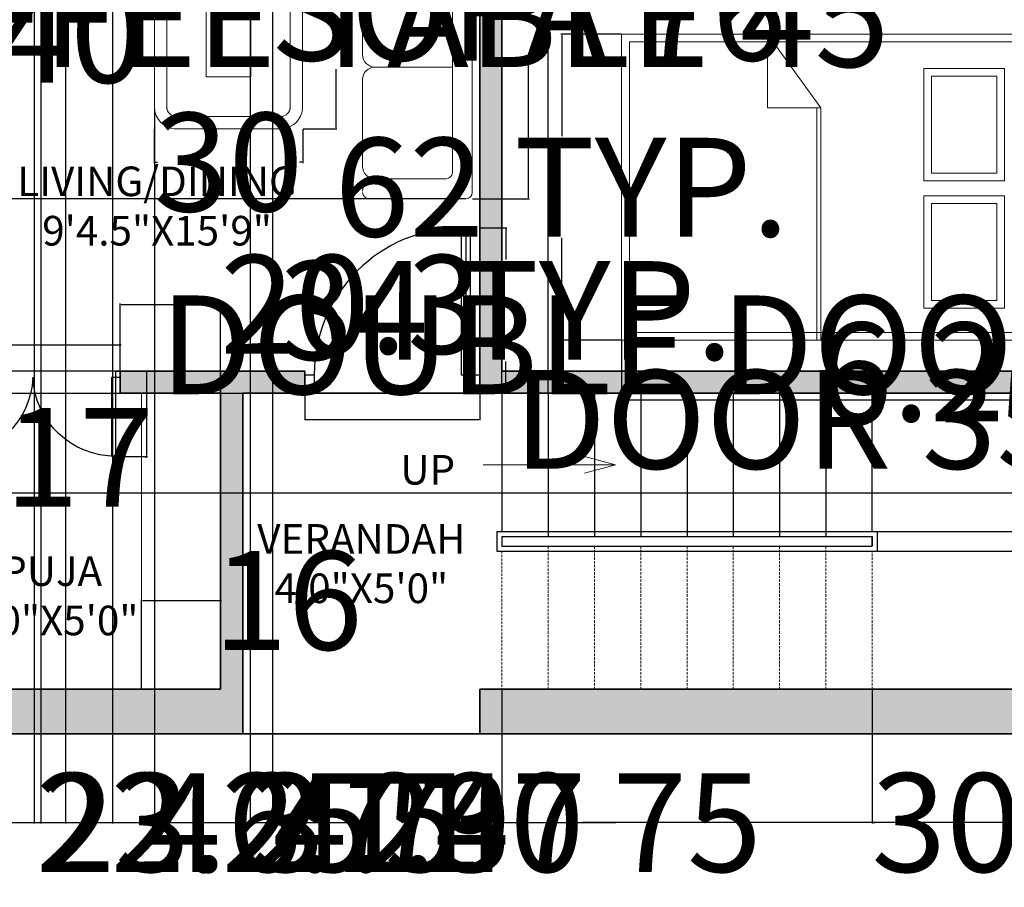
# Model space of a CAD drawing. Units: inches. Extents: x 305 to 776, y 38 to 479.
# Tile 8 of 14: x 419 to 618, y 38 to 214. Entities that reach past the tile are written whole.
import ezdxf

# ---------------------------------------------------------------- set-up
doc = ezdxf.new("R2010")
doc.units = ezdxf.units.IN
doc.header["$MEASUREMENT"] = 0
doc.linetypes.add('DASHED', pattern=[0.75, 0.5, -0.25])
for name, color, linetype, lineweight in [('A-ANNO-DIMS', 2, 'Continuous', 18), ('A-ANNO-SYMB', 3, 'Continuous', 18), ('A-AREA-IDEN', 7, 'Continuous', 18), ('A-DOOR', 4, 'Continuous', 25), ('A-FLOR-CASE', 8, 'Continuous', 20), ('A-FLOR-STRS', 7, 'Continuous', 25), ('A-FLOR-STRS-OVHD', 7, 'DASHED', 18), ('A-FURN', 8, 'Continuous', 18), ('A-WALL', 7, 'Continuous', 35), ('A-WALL-PATT', 252, 'Continuous', 13)]:
    doc.layers.add(name, color=color, linetype=linetype, lineweight=lineweight)
doc.styles.get("Standard").update_dxf_attribs({"font": 'arial.ttf'})
doc.dimstyles.get("Standard").update_dxf_attribs({"dimtxt": 20, "dimasz": 0.18, "dimexe": 0.18, "dimexo": 0.0625, "dimgap": 0.09, "dimtad": 0, "dimtih": 1, "dimtoh": 1, "dimdec": 4, "dimzin": 0, "dimdsep": 46, "dimtxsty": 'Standard', "dimcen": 0.09, "dimadec": 0, "dimazin": 0, "dimtfac": 1, "dimtdec": 4, "dimtofl": 0, "dimtmove": 0, "dimatfit": 3, "dimfxl": 1, "dimtolj": 1, "dimtzin": 0, "dimarcsym": 0})

# ---------------------------------------------------------------- blocks, each defined once
blk = doc.blocks.new('A$C296830DC')
blk.add_line((828.9, 852.6), (828.9, 94.7))
for points in [[(852.6, 94.7), (852.6, 852.6), (805.3, 852.6), (805.3, 94.7)], [(47.4, 94.7), (47.4, 0), (0, 0), (0, 94.7)], [(900, 94.7), (900, 0), (852.6, 0), (852.6, 94.7)]]:
    blk.add_lwpolyline(points, close=True)
blk.add_arc((805.3, 94.7), 757.9, 90, 180)
blk = doc.blocks.new('BED')
for p, q in [((1579.44, 254.58), (1564.49, 243.77)), ((1564.49, 243.77), (1579.44, 254.58)), ((1626.49, 254.58), (1579.44, 254.58)), ((1579.44, 254.58), (1579.44, 243.77)), ((1626.49, 253.76), (1579.44, 253.76)), ((1579.44, 243.77), (1564.49, 243.77))]:
    blk.add_line(p, q)
for points in [[(1626.49, 214.2), (1564.49, 214.2), (1564.49, 294.96), (1626.49, 294.96)], [(1624.92, 215.77), (1566.06, 215.77), (1566.06, 293.39), (1624.92, 293.39)], [(1594.24, 275.39), (1571.42, 275.39), (1571.42, 291.78), (1594.24, 291.78)], [(1620.04, 275.39), (1597.22, 275.39), (1597.22, 291.78), (1620.04, 291.78)], [(1592.67, 276.96), (1572.99, 276.96), (1572.99, 290.21), (1592.67, 290.21)], [(1618.47, 276.96), (1598.79, 276.96), (1598.79, 290.21), (1618.47, 290.21)]]:
    blk.add_lwpolyline(points, close=True)
blk = doc.blocks.new('sofa-25')
at = {"color": 0, "linetype": 'ByBlock'}
for p, q in [((0.5351, 0.5197), (0.124, 0.5197)), ((1.0702, 0.5197), (0.6532, 0.5197)), ((1.5935, 0.5197), (1.1883, 0.5197)), ((-0.0295, 0.0295), (-0.0295, 0.4902)), ((1.7471, 0.0591), (1.7471, 0.4902)), ((0.065, 0.124), (0.065, 0.4607)), ((0.5942, 0.0945), (0.5942, 0.4607)), ((1.1293, 0.0945), (1.1293, 0.4607)), ((1.6526, 0.1181), (1.6526, 0.4607)), ((0.0945, 0.0945), (1.6289, 0.0945)), ((0, 0), (1.688, 0))]:
    blk.add_line(p, q, dxfattribs=at)
for centre, radius, start, end in [((0, 0.4902), 0.0295, 90, 180), ((0.0059, 0.4607), 0.0591, 0, 90), ((0.124, 0.4607), 0.0591, 90, 180), ((0.5351, 0.4607), 0.0591, 0, 90), ((0.6532, 0.4607), 0.0591, 90, 180), ((1.0702, 0.4607), 0.0591, 0, 90), ((1.1883, 0.4607), 0.0591, 90, 180), ((1.5935, 0.4607), 0.0591, 0, 90), ((1.7116, 0.4607), 0.0591, 90, 180), ((1.7175, 0.4902), 0.0295, 0, 90), ((0.0945, 0.124), 0.0295, 180, 270), ((1.6289, 0.1181), 0.0236, 270, 0), ((1.688, 0.0591), 0.0591, 270, 0), ((0, 0.0295), 0.0295, 180, 270)]:
    blk.add_arc(centre, radius, start, end, dxfattribs=at)
blk = doc.blocks.new('carp')
for p, q in [((853.97, 318.32), (853.97, 318.33)), ((857.97, 314.33), (857.96, 314.33))]:
    blk.add_line(p, q)
for points in [[(853.97, 318.33), (831.57, 318.33)], [(853.97, 315.83), (831.57, 315.83)], [(827.97, 314.73), (827.97, 277.33)], [(830.47, 314.73), (830.47, 277.33)], [(855.47, 277.33), (855.47, 314.33)], [(857.97, 277.33), (857.97, 314.33)], [(831.97, 275.83), (853.97, 275.83)], [(831.97, 273.33), (853.97, 273.33)]]:
    blk.add_lwpolyline(points)
blk.add_lwpolyline([(838.47, 307.83), (838.47, 283.83), (847.47, 283.83), (847.47, 307.83)], close=True)
for centre, radius, start, end in [((831.77, 314.53), 3.81, 87.0112, 182.9888), ((853.86, 314.21), 4.11, 358.8861, 88.4626), ((831.77, 314.53), 1.31, 87.0112, 182.9888), ((853.86, 314.21), 1.61, 358.8861, 88.4626), ((832.52, 277.88), 4.59, 186.916, 263.084), ((832.52, 277.88), 2.09, 186.916, 263.084), ((853.42, 277.88), 2.09, 276.916, 353.084), ((853.42, 277.88), 4.59, 276.916, 353.084)]:
    blk.add_arc(centre, radius, start, end)
blk = doc.blocks.new('A$C16FA5A5B')
for p, q in [((50, 487.5), (25, 487.5)), ((25, 487.5), (25, 37.5)), ((50, 37.5), (50, 487.5)), ((950, 37.5), (950, 487.5)), ((950, 487.5), (975, 487.5)), ((975, 487.5), (975, 37.5)), ((0, 0), (0, 37.5)), ((0, 37.5), (25, 37.5)), ((25, 0), (0, 0)), ((25, 37.5), (25, 0)), ((25, 37.5), (50, 37.5)), ((975, 37.5), (950, 37.5)), ((975, 37.5), (975, 0)), ((1000, 37.5), (975, 37.5)), ((975, 0), (1000, 0)), ((1000, 0), (1000, 37.5))]:
    blk.add_line(p, q)
for centre, start, end in [((28.6, 15.6), 2.662, 90.4344), ((971.4, 15.6), 89.5656, 177.338)]:
    blk.add_arc(centre, 471.9, start, end)
blk = doc.blocks.new('*D17')
at = {"layer": 'A-ANNO-DIMS', "color": 0, "lineweight": -2, "transparency": 16777216}
for p, q in [((476.73, 138.32), (476.73, 132.89)), ((512.13, 138.32), (512.13, 132.89)), ((476.91, 133.07), (511.95, 133.07)), ((512.13, 133.07), (512.31, 133.07))]:
    blk.add_line(p, q, dxfattribs=at)
at = {"layer": 'A-ANNO-DIMS', "color": 0, "transparency": 16777216}
for points in [[(476.91, 133.1), (476.91, 133.04), (476.73, 133.07)], [(511.95, 133.1), (511.95, 133.04), (512.13, 133.07)]]:
    blk.add_solid(points, dxfattribs=at)
at = {"layer": 'Defpoints', "color": 0, "transparency": 16777216}
for p in [(476.73, 138.38), (512.13, 138.38), (512.13, 133.07)]:
    blk.add_point(p, dxfattribs=at)
at = {"layer": 'A-ANNO-DIMS', "color": 0, "transparency": 16777216, "insert": (606.37, 133.07), "char_height": 20, "attachment_point": 5}
blk.add_mtext('\\A1;DOOR 35 TYP.', dxfattribs=at)
blk = doc.blocks.new('*D18')
at = {"layer": 'A-ANNO-DIMS', "color": 0, "lineweight": -2, "transparency": 16777216}
for p, q in [((512.2, 171.92), (517.62, 171.92)), ((517.44, 171.74), (517.44, 165.46)), ((517.44, 138.56), (517.44, 144.84)), ((512.2, 138.38), (517.62, 138.38))]:
    blk.add_line(p, q, dxfattribs=at)
at = {"layer": 'A-ANNO-DIMS', "color": 0, "transparency": 16777216}
for points in [[(517.41, 171.74), (517.47, 171.74), (517.44, 171.92)], [(517.41, 138.56), (517.47, 138.56), (517.44, 138.38)]]:
    blk.add_solid(points, dxfattribs=at)
at = {"layer": 'Defpoints', "color": 0, "transparency": 16777216}
for p in [(512.13, 171.92), (517.44, 171.92), (512.13, 138.38)]:
    blk.add_point(p, dxfattribs=at)
at = {"layer": 'A-ANNO-DIMS', "color": 0, "transparency": 16777216, "insert": (517.44, 155.15), "char_height": 20, "attachment_point": 5}
blk.add_mtext('\\A1;34 TYP.', dxfattribs=at)
blk = doc.blocks.new('*D19')
at = {"layer": 'A-ANNO-DIMS', "color": 0, "lineweight": -2, "transparency": 16777216}
for p, q in [((557.63, 250.82), (557.63, 245.98)), ((589.13, 250.82), (589.13, 245.98)), ((557.63, 246.16), (557.45, 246.16)), ((588.95, 246.16), (557.81, 246.16))]:
    blk.add_line(p, q, dxfattribs=at)
at = {"layer": 'A-ANNO-DIMS', "color": 0, "transparency": 16777216}
for points in [[(557.81, 246.19), (557.81, 246.13), (557.63, 246.16)], [(588.95, 246.19), (588.95, 246.13), (589.13, 246.16)]]:
    blk.add_solid(points, dxfattribs=at)
at = {"layer": 'Defpoints', "color": 0, "transparency": 16777216}
for p in [(557.63, 250.88), (589.13, 250.88), (557.63, 246.16)]:
    blk.add_point(p, dxfattribs=at)
at = {"layer": 'A-ANNO-DIMS', "color": 0, "transparency": 16777216, "insert": (463.39, 246.16), "char_height": 20, "attachment_point": 5}
blk.add_mtext('\\A1;DOOR 32 TYP.', dxfattribs=at)
blk = doc.blocks.new('*D21')
at = {"layer": 'A-ANNO-DIMS', "color": 0, "lineweight": -2, "transparency": 16777216}
for p, q in [((403.93, 142.94), (403.93, 148.37)), ((404.11, 148.19), (439.15, 148.19)), ((439.33, 142.94), (439.33, 148.37)), ((439.33, 148.19), (439.51, 148.19))]:
    blk.add_line(p, q, dxfattribs=at)
at = {"layer": 'A-ANNO-DIMS', "color": 0, "transparency": 16777216}
for points in [[(404.11, 148.22), (404.11, 148.16), (403.93, 148.19)], [(439.15, 148.22), (439.15, 148.16), (439.33, 148.19)]]:
    blk.add_solid(points, dxfattribs=at)
at = {"layer": 'Defpoints', "color": 0, "transparency": 16777216}
for p in [(439.33, 148.19), (403.93, 142.88), (439.33, 142.88)]:
    blk.add_point(p, dxfattribs=at)
at = {"layer": 'A-ANNO-DIMS', "color": 0, "transparency": 16777216, "insert": (560.63, 148.19), "char_height": 20, "attachment_point": 5}
blk.add_mtext('\\A1;DOUBLE DOOR 35', dxfattribs=at)
blk = doc.blocks.new('*D22')
at = {"layer": 'A-ANNO-DIMS', "color": 0, "lineweight": -2, "transparency": 16777216}
for p, q in [((439.4, 142.88), (444.82, 142.88)), ((444.64, 142.7), (444.64, 125.74)), ((439.4, 125.56), (444.82, 125.56)), ((444.64, 125.38), (444.46, 125.38)), ((444.64, 125.56), (444.64, 125.38))]:
    blk.add_line(p, q, dxfattribs=at)
at = {"layer": 'A-ANNO-DIMS', "color": 0, "transparency": 16777216}
for points in [[(444.61, 142.7), (444.67, 142.7), (444.64, 142.88)], [(444.61, 125.74), (444.67, 125.74), (444.64, 125.56)]]:
    blk.add_solid(points, dxfattribs=at)
at = {"layer": 'Defpoints', "color": 0, "transparency": 16777216}
for p in [(439.33, 142.88), (439.33, 125.56), (444.64, 125.56)]:
    blk.add_point(p, dxfattribs=at)
at = {"layer": 'A-ANNO-DIMS', "color": 0, "transparency": 16777216, "insert": (430.99, 125.38), "char_height": 20, "attachment_point": 5}
blk.add_mtext('\\A1;17', dxfattribs=at)
blk = doc.blocks.new('*D29')
at = {"layer": 'A-ANNO-DIMS', "color": 0, "lineweight": -2, "transparency": 16777216}
for p, q in [((540.87, 149.08), (540.87, 136.85)), ((621.63, 149.08), (621.63, 136.85)), ((541.05, 137.03), (621.45, 137.03)), ((621.63, 137.03), (621.81, 137.03))]:
    blk.add_line(p, q, dxfattribs=at)
at = {"layer": 'A-ANNO-DIMS', "color": 0, "transparency": 16777216}
for points in [[(541.05, 137.06), (541.05, 137), (540.87, 137.03)], [(621.45, 137.06), (621.45, 137), (621.63, 137.03)]]:
    blk.add_solid(points, dxfattribs=at)
at = {"layer": 'Defpoints', "color": 0, "transparency": 16777216}
for p in [(540.87, 149.14), (621.63, 149.14), (621.63, 137.03)]:
    blk.add_point(p, dxfattribs=at)
at = {"layer": 'A-ANNO-DIMS', "color": 0, "transparency": 16777216, "insert": (702.74, 137.03), "char_height": 20, "attachment_point": 5}
blk.add_mtext('\\A1;BED 81 TYP.', dxfattribs=at)
blk = doc.blocks.new('*D30')
at = {"layer": 'A-ANNO-DIMS', "color": 0, "lineweight": -2, "transparency": 16777216}
for p, q in [((540.81, 211.14), (528.58, 211.14)), ((528.76, 210.96), (528.76, 190.45)), ((528.76, 149.32), (528.76, 169.84)), ((540.81, 149.14), (528.58, 149.14))]:
    blk.add_line(p, q, dxfattribs=at)
at = {"layer": 'A-ANNO-DIMS', "color": 0, "transparency": 16777216}
for points in [[(528.73, 210.96), (528.79, 210.96), (528.76, 211.14)], [(528.73, 149.32), (528.79, 149.32), (528.76, 149.14)]]:
    blk.add_solid(points, dxfattribs=at)
at = {"layer": 'Defpoints', "color": 0, "transparency": 16777216}
for p in [(540.87, 211.14), (528.76, 149.14), (540.87, 149.14)]:
    blk.add_point(p, dxfattribs=at)
at = {"layer": 'A-ANNO-DIMS', "color": 0, "transparency": 16777216, "insert": (528.76, 180.14), "char_height": 20, "attachment_point": 5}
blk.add_mtext('\\A1;62 TYP.', dxfattribs=at)
blk = doc.blocks.new('*D35')
at = {"layer": 'A-ANNO-DIMS', "color": 0, "lineweight": -2, "transparency": 16777216}
for p, q in [((510.7, 253.8), (522.21, 253.8)), ((522.03, 253.62), (522.03, 226.23)), ((522.03, 177.97), (522.03, 205.36)), ((510.7, 177.79), (522.21, 177.79))]:
    blk.add_line(p, q, dxfattribs=at)
at = {"layer": 'A-ANNO-DIMS', "color": 0, "transparency": 16777216}
for points in [[(522, 253.62), (522.06, 253.62), (522.03, 253.8)], [(522, 177.97), (522.06, 177.97), (522.03, 177.79)]]:
    blk.add_solid(points, dxfattribs=at)
at = {"layer": 'Defpoints', "color": 0, "transparency": 16777216}
for p in [(510.63, 253.8), (522.03, 253.8), (510.63, 177.79)]:
    blk.add_point(p, dxfattribs=at)
at = {"layer": 'A-ANNO-DIMS', "color": 0, "transparency": 16777216, "insert": (522.03, 215.8), "char_height": 20, "attachment_point": 5}
blk.add_mtext('\\A1;SOFA 76', dxfattribs=at)
blk = doc.blocks.new('*D37')
at = {"layer": 'A-ANNO-DIMS', "color": 0, "lineweight": -2, "transparency": 16777216}
for p, q in [((476.35, 237.03), (483.22, 237.03)), ((483.04, 236.85), (483.04, 224.94)), ((483.04, 192.15), (483.04, 204.06)), ((476.35, 191.97), (483.22, 191.97))]:
    blk.add_line(p, q, dxfattribs=at)
at = {"layer": 'A-ANNO-DIMS', "color": 0, "transparency": 16777216}
for points in [[(483.01, 236.85), (483.07, 236.85), (483.04, 237.03)], [(483.01, 192.15), (483.07, 192.15), (483.04, 191.97)]]:
    blk.add_solid(points, dxfattribs=at)
at = {"layer": 'Defpoints', "color": 0, "transparency": 16777216}
for p in [(476.28, 237.03), (483.04, 237.03), (476.28, 191.97)]:
    blk.add_point(p, dxfattribs=at)
at = {"layer": 'A-ANNO-DIMS', "color": 0, "transparency": 16777216, "insert": (483.04, 214.5), "char_height": 20, "attachment_point": 5}
blk.add_mtext('\\A1;COFFEE TABLE 45', dxfattribs=at)
blk = doc.blocks.new('*D38')
at = {"layer": 'A-ANNO-DIMS', "color": 0, "lineweight": -2, "transparency": 16777216}
for p, q in [((446.19, 191.91), (446.19, 185.03)), ((476.28, 191.91), (476.28, 185.03)), ((446.37, 185.21), (446.86, 185.21)), ((476.1, 185.21), (475.61, 185.21))]:
    blk.add_line(p, q, dxfattribs=at)
at = {"layer": 'A-ANNO-DIMS', "color": 0, "transparency": 16777216}
for points in [[(446.37, 185.24), (446.37, 185.18), (446.19, 185.21)], [(476.1, 185.24), (476.1, 185.18), (476.28, 185.21)]]:
    blk.add_solid(points, dxfattribs=at)
at = {"layer": 'Defpoints', "color": 0, "transparency": 16777216}
for p in [(446.19, 191.97), (476.28, 191.97), (476.28, 185.21)]:
    blk.add_point(p, dxfattribs=at)
at = {"layer": 'A-ANNO-DIMS', "color": 0, "transparency": 16777216, "insert": (461.24, 185.21), "char_height": 20, "attachment_point": 5}
blk.add_mtext('\\A1;30', dxfattribs=at)
blk = doc.blocks.new('*D39')
at = {"layer": 'A-ANNO-DIMS', "color": 0, "lineweight": -2, "transparency": 16777216}
for p, q in [((404.2, 231.29), (410.31, 231.29)), ((410.13, 231.11), (410.13, 221.59)), ((410.13, 191.47), (410.13, 200.99)), ((404.2, 191.29), (410.31, 191.29))]:
    blk.add_line(p, q, dxfattribs=at)
at = {"layer": 'A-ANNO-DIMS', "color": 0, "transparency": 16777216}
for points in [[(410.1, 231.11), (410.16, 231.11), (410.13, 231.29)], [(410.1, 191.47), (410.16, 191.47), (410.13, 191.29)]]:
    blk.add_solid(points, dxfattribs=at)
at = {"layer": 'Defpoints', "color": 0, "transparency": 16777216}
for p in [(404.13, 231.29), (410.13, 231.29), (404.13, 191.29)]:
    blk.add_point(p, dxfattribs=at)
at = {"layer": 'A-ANNO-DIMS', "color": 0, "transparency": 16777216, "insert": (410.13, 211.29), "char_height": 20, "attachment_point": 5}
blk.add_mtext('\\A1;TV 40', dxfattribs=at)
blk = doc.blocks.new('*D45')
at = {"layer": 'A-ANNO-DIMS', "color": 0, "lineweight": -2, "transparency": 16777216}
for p, q in [((390.63, 69.32), (390.63, 51.2)), ((630.63, 69.32), (630.63, 51.2)), ((390.81, 51.38), (488.31, 51.38)), ((630.45, 51.38), (532.95, 51.38))]:
    blk.add_line(p, q, dxfattribs=at)
at = {"layer": 'A-ANNO-DIMS', "color": 0, "transparency": 16777216}
for points in [[(390.81, 51.41), (390.81, 51.35), (390.63, 51.38)], [(630.45, 51.41), (630.45, 51.35), (630.63, 51.38)]]:
    blk.add_solid(points, dxfattribs=at)
at = {"layer": 'Defpoints', "color": 0, "transparency": 16777216}
for p in [(390.63, 69.38), (630.63, 69.38), (630.63, 51.38)]:
    blk.add_point(p, dxfattribs=at)
at = {"layer": 'A-ANNO-DIMS', "color": 0, "transparency": 16777216, "insert": (510.63, 51.38), "char_height": 20, "attachment_point": 5}
blk.add_mtext('\\A1;240', dxfattribs=at)
blk = doc.blocks.new('*D47')
at = {"layer": 'A-ANNO-DIMS', "color": 0, "lineweight": -2, "transparency": 16777216}
for p, q in [((465.63, 331.82), (465.63, 51.2)), ((470.13, 331.82), (470.13, 51.2)), ((465.81, 51.38), (469.95, 51.38)), ((470.13, 51.38), (470.31, 51.38))]:
    blk.add_line(p, q, dxfattribs=at)
at = {"layer": 'A-ANNO-DIMS', "color": 0, "transparency": 16777216}
for points in [[(465.81, 51.41), (465.81, 51.35), (465.63, 51.38)], [(469.95, 51.41), (469.95, 51.35), (470.13, 51.38)]]:
    blk.add_solid(points, dxfattribs=at)
at = {"layer": 'Defpoints', "color": 0, "transparency": 16777216}
for p in [(465.63, 331.88), (470.13, 331.88), (470.13, 51.38)]:
    blk.add_point(p, dxfattribs=at)
at = {"layer": 'A-ANNO-DIMS', "color": 0, "transparency": 16777216, "insert": (489.09, 51.38), "char_height": 20, "attachment_point": 5}
blk.add_mtext('\\A1;4.5', dxfattribs=at)
blk = doc.blocks.new('*D48')
at = {"layer": 'A-ANNO-DIMS', "color": 0, "lineweight": -2, "transparency": 16777216}
for p, q in [((404, 138.38), (648.81, 138.38)), ((648.63, 138.38), (648.63, 138.56)), ((648.63, 138.56), (648.81, 138.56)), ((648.63, 118.36), (648.63, 138.2)), ((399.7, 118.18), (648.81, 118.18))]:
    blk.add_line(p, q, dxfattribs=at)
at = {"layer": 'A-ANNO-DIMS', "color": 0, "transparency": 16777216}
for points in [[(648.6, 138.2), (648.66, 138.2), (648.63, 138.38)], [(648.6, 118.36), (648.66, 118.36), (648.63, 118.18)]]:
    blk.add_solid(points, dxfattribs=at)
at = {"layer": 'Defpoints', "color": 0, "transparency": 16777216}
for p in [(403.93, 138.38), (648.63, 138.38), (399.63, 118.18)]:
    blk.add_point(p, dxfattribs=at)
at = {"layer": 'A-ANNO-DIMS', "color": 0, "transparency": 16777216, "insert": (674.95, 138.56), "char_height": 20, "attachment_point": 5}
blk.add_mtext('\\A1;20.2', dxfattribs=at)
blk = doc.blocks.new('*D55')
at = {"layer": 'A-ANNO-DIMS', "color": 0, "lineweight": -2, "transparency": 16777216}
for p, q in [((516.63, 78.32), (516.63, 51.2)), ((591.63, 78.32), (591.63, 51.2)), ((516.81, 51.38), (539.73, 51.38)), ((591.45, 51.38), (568.54, 51.38))]:
    blk.add_line(p, q, dxfattribs=at)
at = {"layer": 'A-ANNO-DIMS', "color": 0, "transparency": 16777216}
for points in [[(516.81, 51.41), (516.81, 51.35), (516.63, 51.38)], [(591.45, 51.41), (591.45, 51.35), (591.63, 51.38)]]:
    blk.add_solid(points, dxfattribs=at)
at = {"layer": 'Defpoints', "color": 0, "transparency": 16777216}
for p in [(516.63, 78.38), (591.63, 78.38), (591.63, 51.38)]:
    blk.add_point(p, dxfattribs=at)
at = {"layer": 'A-ANNO-DIMS', "color": 0, "transparency": 16777216, "insert": (554.13, 51.38), "char_height": 20, "attachment_point": 5}
blk.add_mtext('\\A1;75', dxfattribs=at)
blk = doc.blocks.new('*D56')
at = {"layer": 'A-ANNO-DIMS', "color": 0, "lineweight": -2, "transparency": 16777216}
for p, q in [((591.63, 78.32), (591.63, 51.2)), ((621.63, 78.32), (621.63, 51.2)), ((591.81, 51.38), (592.26, 51.38)), ((621.45, 51.38), (621.01, 51.38))]:
    blk.add_line(p, q, dxfattribs=at)
at = {"layer": 'A-ANNO-DIMS', "color": 0, "transparency": 16777216}
for points in [[(591.81, 51.41), (591.81, 51.35), (591.63, 51.38)], [(621.45, 51.41), (621.45, 51.35), (621.63, 51.38)]]:
    blk.add_solid(points, dxfattribs=at)
at = {"layer": 'Defpoints', "color": 0, "transparency": 16777216}
for p in [(591.63, 78.38), (621.63, 78.38), (621.63, 51.38)]:
    blk.add_point(p, dxfattribs=at)
at = {"layer": 'A-ANNO-DIMS', "color": 0, "transparency": 16777216, "insert": (606.63, 51.38), "char_height": 20, "attachment_point": 5}
blk.add_mtext('\\A1;30', dxfattribs=at)
blk = doc.blocks.new('*D57')
at = {"layer": 'A-ANNO-DIMS', "color": 0, "lineweight": -2, "transparency": 16777216}
for p, q in [((591.7, 138.38), (648.81, 138.38)), ((648.63, 138.2), (648.63, 134.68)), ((648.63, 110.56), (648.63, 114.08)), ((591.7, 110.38), (648.81, 110.38))]:
    blk.add_line(p, q, dxfattribs=at)
at = {"layer": 'A-ANNO-DIMS', "color": 0, "transparency": 16777216}
for points in [[(648.6, 138.2), (648.66, 138.2), (648.63, 138.38)], [(648.6, 110.56), (648.66, 110.56), (648.63, 110.38)]]:
    blk.add_solid(points, dxfattribs=at)
at = {"layer": 'Defpoints', "color": 0, "transparency": 16777216}
for p in [(591.63, 138.38), (591.63, 110.38), (648.63, 110.38)]:
    blk.add_point(p, dxfattribs=at)
at = {"layer": 'A-ANNO-DIMS', "color": 0, "transparency": 16777216, "insert": (648.63, 124.38), "char_height": 20, "attachment_point": 5}
blk.add_mtext('\\A1;28', dxfattribs=at)
blk = doc.blocks.new('*D58')
at = {"layer": 'A-ANNO-DIMS', "color": 0, "lineweight": -2, "transparency": 16777216}
for p, q in [((516.63, 138.44), (516.63, 447.56)), ((516.81, 447.38), (525.83, 447.38)), ((526.01, 138.44), (526.01, 447.56)), ((526.01, 447.38), (526.19, 447.38))]:
    blk.add_line(p, q, dxfattribs=at)
at = {"layer": 'A-ANNO-DIMS', "color": 0, "transparency": 16777216}
for points in [[(516.81, 447.41), (516.81, 447.35), (516.63, 447.38)], [(525.83, 447.41), (525.83, 447.35), (526.01, 447.38)]]:
    blk.add_solid(points, dxfattribs=at)
at = {"layer": 'Defpoints', "color": 0, "transparency": 16777216}
for p in [(526.01, 447.38), (516.63, 138.38), (526.01, 138.38)]:
    blk.add_point(p, dxfattribs=at)
at = {"layer": 'A-ANNO-DIMS', "color": 0, "transparency": 16777216, "insert": (560.1, 447.38), "char_height": 20, "attachment_point": 5}
blk.add_mtext('\\A1;9.375', dxfattribs=at)
blk = doc.blocks.new('*D59')
at = {"layer": 'A-ANNO-DIMS', "color": 0, "lineweight": -2, "transparency": 16777216}
for p, q in [((591.7, 110.38), (648.81, 110.38)), ((648.63, 110.38), (648.63, 110.56)), ((648.63, 110.56), (648.81, 110.56)), ((648.63, 106.56), (648.63, 110.2)), ((591.7, 106.38), (648.81, 106.38))]:
    blk.add_line(p, q, dxfattribs=at)
at = {"layer": 'A-ANNO-DIMS', "color": 0, "transparency": 16777216}
for points in [[(648.6, 110.2), (648.66, 110.2), (648.63, 110.38)], [(648.6, 106.56), (648.66, 106.56), (648.63, 106.38)]]:
    blk.add_solid(points, dxfattribs=at)
at = {"layer": 'Defpoints', "color": 0, "transparency": 16777216}
for p in [(591.63, 110.38), (648.63, 110.38), (591.63, 106.38)]:
    blk.add_point(p, dxfattribs=at)
at = {"layer": 'A-ANNO-DIMS', "color": 0, "transparency": 16777216, "insert": (655.82, 110.56), "char_height": 20, "attachment_point": 5}
blk.add_mtext('\\A1;4', dxfattribs=at)
blk = doc.blocks.new('*D60')
at = {"layer": 'A-ANNO-DIMS', "color": 0, "lineweight": -2, "transparency": 16777216}
for p, q in [((428.26, 331.82), (428.26, 51.2)), ((465.63, 331.82), (465.63, 51.2)), ((428.44, 51.38), (465.45, 51.38)), ((465.63, 51.38), (465.81, 51.38))]:
    blk.add_line(p, q, dxfattribs=at)
at = {"layer": 'A-ANNO-DIMS', "color": 0, "transparency": 16777216}
for points in [[(428.44, 51.41), (428.44, 51.35), (428.26, 51.38)], [(465.45, 51.41), (465.45, 51.35), (465.63, 51.38)]]:
    blk.add_solid(points, dxfattribs=at)
at = {"layer": 'Defpoints', "color": 0, "transparency": 16777216}
for p in [(428.26, 331.88), (465.63, 331.88), (465.63, 51.38)]:
    blk.add_point(p, dxfattribs=at)
at = {"layer": 'A-ANNO-DIMS', "color": 0, "transparency": 16777216, "insert": (499.64, 51.38), "char_height": 20, "attachment_point": 5}
blk.add_mtext('\\A1;37.37', dxfattribs=at)
blk = doc.blocks.new('*D61')
at = {"layer": 'A-ANNO-DIMS', "color": 0, "lineweight": -2, "transparency": 16777216}
for p, q in [((437.73, 398.69), (437.73, 51.2)), ((465.63, 398.69), (465.63, 51.2)), ((437.91, 51.38), (465.45, 51.38)), ((465.63, 51.38), (465.81, 51.38))]:
    blk.add_line(p, q, dxfattribs=at)
at = {"layer": 'A-ANNO-DIMS', "color": 0, "transparency": 16777216}
for points in [[(437.91, 51.41), (437.91, 51.35), (437.73, 51.38)], [(465.45, 51.41), (465.45, 51.35), (465.63, 51.38)]]:
    blk.add_solid(points, dxfattribs=at)
at = {"layer": 'Defpoints', "color": 0, "transparency": 16777216}
for p in [(437.73, 398.75), (465.63, 398.75), (465.63, 51.38)]:
    blk.add_point(p, dxfattribs=at)
at = {"layer": 'A-ANNO-DIMS', "color": 0, "transparency": 16777216, "insert": (492.07, 51.38), "char_height": 20, "attachment_point": 5}
blk.add_mtext('\\A1;27.9', dxfattribs=at)
blk = doc.blocks.new('*D62')
at = {"layer": 'A-ANNO-DIMS', "color": 0, "lineweight": -2, "transparency": 16777216}
for p, q in [((399.63, 336.32), (399.63, 51.2)), ((423.23, 336.32), (423.23, 51.2)), ((399.81, 51.38), (423.05, 51.38)), ((423.23, 51.38), (423.41, 51.38))]:
    blk.add_line(p, q, dxfattribs=at)
at = {"layer": 'A-ANNO-DIMS', "color": 0, "transparency": 16777216}
for points in [[(399.81, 51.41), (399.81, 51.35), (399.63, 51.38)], [(423.05, 51.41), (423.05, 51.35), (423.23, 51.38)]]:
    blk.add_solid(points, dxfattribs=at)
at = {"layer": 'Defpoints', "color": 0, "transparency": 16777216}
for p in [(399.63, 336.38), (423.23, 336.38), (423.23, 51.38)]:
    blk.add_point(p, dxfattribs=at)
at = {"layer": 'A-ANNO-DIMS', "color": 0, "transparency": 16777216, "insert": (449.64, 51.38), "char_height": 20, "attachment_point": 5}
blk.add_mtext('\\A1;23.6', dxfattribs=at)
blk = doc.blocks.new('*D65')
at = {"layer": 'A-ANNO-DIMS', "color": 0, "lineweight": -2, "transparency": 16777216}
for p, q in [((399.63, 351.22), (399.63, 51.2)), ((421.89, 351.22), (421.89, 51.2)), ((399.81, 51.38), (421.71, 51.38)), ((421.89, 51.38), (422.07, 51.38))]:
    blk.add_line(p, q, dxfattribs=at)
at = {"layer": 'A-ANNO-DIMS', "color": 0, "transparency": 16777216}
for points in [[(399.81, 51.41), (399.81, 51.35), (399.63, 51.38)], [(421.71, 51.41), (421.71, 51.35), (421.89, 51.38)]]:
    blk.add_solid(points, dxfattribs=at)
at = {"layer": 'Defpoints', "color": 0, "transparency": 16777216}
for p in [(399.63, 351.28), (421.89, 351.28), (421.89, 51.38)]:
    blk.add_point(p, dxfattribs=at)
at = {"layer": 'A-ANNO-DIMS', "color": 0, "transparency": 16777216, "insert": (463.84, 51.38), "char_height": 20, "attachment_point": 5}
blk.add_mtext('\\A1;22.257', dxfattribs=at)
blk = doc.blocks.new('*D67')
at = {"layer": 'A-ANNO-DIMS', "color": 0, "lineweight": -2, "transparency": 16777216}
for p, q in [((439.33, 138.44), (439.33, 156.56)), ((439.51, 156.38), (459.45, 156.38)), ((459.63, 138.44), (459.63, 156.56)), ((459.63, 156.38), (459.81, 156.38))]:
    blk.add_line(p, q, dxfattribs=at)
at = {"layer": 'A-ANNO-DIMS', "color": 0, "transparency": 16777216}
for points in [[(439.51, 156.41), (439.51, 156.35), (439.33, 156.38)], [(459.45, 156.41), (459.45, 156.35), (459.63, 156.38)]]:
    blk.add_solid(points, dxfattribs=at)
at = {"layer": 'Defpoints', "color": 0, "transparency": 16777216}
for p in [(459.63, 156.38), (439.33, 138.38), (459.63, 138.38)]:
    blk.add_point(p, dxfattribs=at)
at = {"layer": 'A-ANNO-DIMS', "color": 0, "transparency": 16777216, "insert": (486.05, 156.38), "char_height": 20, "attachment_point": 5}
blk.add_mtext('\\A1;20.3', dxfattribs=at)
blk = doc.blocks.new('*D69')
at = {"layer": 'A-ANNO-DIMS', "color": 0, "lineweight": -2, "transparency": 16777216}
for p, q in [((621.7, 149.14), (648.81, 149.14)), ((648.63, 148.96), (648.63, 143.06)), ((621.7, 142.88), (648.81, 142.88)), ((648.63, 142.7), (648.45, 142.7)), ((648.63, 142.88), (648.63, 142.7))]:
    blk.add_line(p, q, dxfattribs=at)
at = {"layer": 'A-ANNO-DIMS', "color": 0, "transparency": 16777216}
for points in [[(648.6, 148.96), (648.66, 148.96), (648.63, 149.14)], [(648.6, 143.06), (648.66, 143.06), (648.63, 142.88)]]:
    blk.add_solid(points, dxfattribs=at)
at = {"layer": 'Defpoints', "color": 0, "transparency": 16777216}
for p in [(621.63, 149.14), (621.63, 142.88), (648.63, 142.88)]:
    blk.add_point(p, dxfattribs=at)
at = {"layer": 'A-ANNO-DIMS', "color": 0, "transparency": 16777216, "insert": (614.67, 142.7), "char_height": 20, "attachment_point": 5}
blk.add_mtext('\\A1;6.262', dxfattribs=at)
blk = doc.blocks.new('*D70')
at = {"layer": 'A-ANNO-DIMS', "color": 0, "lineweight": -2, "transparency": 16777216}
for p, q in [((443.63, 78.44), (443.63, 96.56)), ((443.81, 96.38), (459.45, 96.38)), ((459.63, 78.44), (459.63, 96.56)), ((459.63, 96.38), (459.81, 96.38))]:
    blk.add_line(p, q, dxfattribs=at)
at = {"layer": 'A-ANNO-DIMS', "color": 0, "transparency": 16777216}
for points in [[(443.81, 96.41), (443.81, 96.35), (443.63, 96.38)], [(459.45, 96.41), (459.45, 96.35), (459.63, 96.38)]]:
    blk.add_solid(points, dxfattribs=at)
at = {"layer": 'Defpoints', "color": 0, "transparency": 16777216}
for p in [(459.63, 96.38), (443.63, 78.38), (459.63, 78.38)]:
    blk.add_point(p, dxfattribs=at)
at = {"layer": 'A-ANNO-DIMS', "color": 0, "transparency": 16777216, "insert": (473.28, 96.38), "char_height": 20, "attachment_point": 5}
blk.add_mtext('\\A1;16', dxfattribs=at)
blk = doc.blocks.new('*D72')
at = {"layer": 'A-ANNO-DIMS', "color": 0, "lineweight": -2, "transparency": 16777216}
for p, q in [((446.24, 195.91), (446.24, 51.2)), ((404.13, 191.23), (404.13, 51.2)), ((404.31, 51.38), (446.06, 51.38)), ((446.24, 51.38), (446.42, 51.38))]:
    blk.add_line(p, q, dxfattribs=at)
at = {"layer": 'A-ANNO-DIMS', "color": 0, "transparency": 16777216}
for points in [[(404.31, 51.41), (404.31, 51.35), (404.13, 51.38)], [(446.06, 51.41), (446.06, 51.35), (446.24, 51.38)]]:
    blk.add_solid(points, dxfattribs=at)
at = {"layer": 'Defpoints', "color": 0, "transparency": 16777216}
for p in [(446.24, 195.97), (404.13, 191.29), (446.24, 51.38)]:
    blk.add_point(p, dxfattribs=at)
at = {"layer": 'A-ANNO-DIMS', "color": 0, "transparency": 16777216, "insert": (478.73, 51.38), "char_height": 20, "attachment_point": 5}
blk.add_mtext('\\A1;42.11', dxfattribs=at)
blk = doc.blocks.new('*D73')
at = {"layer": 'A-ANNO-DIMS', "color": 0, "lineweight": -2, "transparency": 16777216}
for p, q in [((509.31, 177.79), (372.45, 177.79)), ((372.63, 177.61), (372.63, 170.64)), ((372.63, 143.06), (372.63, 150.03)), ((476.67, 142.88), (372.45, 142.88))]:
    blk.add_line(p, q, dxfattribs=at)
at = {"layer": 'A-ANNO-DIMS', "color": 0, "transparency": 16777216}
for points in [[(372.6, 177.61), (372.66, 177.61), (372.63, 177.79)], [(372.6, 143.06), (372.66, 143.06), (372.63, 142.88)]]:
    blk.add_solid(points, dxfattribs=at)
at = {"layer": 'Defpoints', "color": 0, "transparency": 16777216}
for p in [(509.37, 177.79), (372.63, 142.88), (476.73, 142.88)]:
    blk.add_point(p, dxfattribs=at)
at = {"layer": 'A-ANNO-DIMS', "color": 0, "transparency": 16777216, "insert": (372.63, 160.34), "char_height": 20, "attachment_point": 5}
blk.add_mtext('\\A1;34.91', dxfattribs=at)

msp = doc.modelspace()

# ---------------------------------------------------------------- hatches: boundary and pattern name
at = {"layer": 'A-WALL-PATT'}
h = msp.add_hatch(color=256, dxfattribs=at)
h.dxf.hatch_style = 1
h.paths.add_polyline_path([(481.3329, 429.382), (390.6329, 429.382), (390.6329, 398.067), (399.6329, 398.067), (399.6329, 420.382), (465.6329, 420.382), (465.6329, 331.882), (470.1329, 331.882), (470.1329, 355.882), (512.1329, 355.882), (512.1329, 337.282), (512.1329, 337.282), (515.8592, 337.282), (516.6329, 337.282), (516.6329, 360.382), (513.3171, 360.382), (470.1329, 360.382), (470.1329, 420.382), (481.3329, 420.382)])
h.paths.add_polyline_path([(630.6329, 429.382), (500.9329, 429.382), (500.9329, 420.382), (502.8693, 420.382), (512.1329, 420.382), (512.1329, 391.882), (516.6329, 391.882), (516.6329, 420.382), (621.6329, 420.382), (621.6329, 388.182), (630.6329, 388.182)])
h.paths.add_polyline_path([(630.6329, 329.382), (621.6329, 329.382), (621.6329, 301.882), (512.1329, 301.882), (512.1329, 297.382), (515.8592, 297.382), (557.6329, 297.382), (621.6329, 297.382), (621.6329, 286.182), (630.6329, 286.182)])
h.paths.add_polyline_path([(630.6329, 266.582), (621.6329, 266.582), (621.6329, 255.382), (589.1329, 255.382), (589.1329, 250.882), (621.6329, 250.882), (621.6329, 226.282), (630.6329, 226.282)])
h.paths.add_polyline_path([(630.6329, 167.482), (621.6329, 167.482), (621.6329, 149.1444), (621.6329, 142.882), (516.6329, 142.882), (516.6329, 261.982), (512.1329, 261.982), (512.1329, 138.382), (621.6329, 138.382), (621.6329, 78.382), (512.1329, 78.382), (512.1329, 69.382), (630.6329, 69.382)])
h.paths.add_polyline_path([(464.1329, 138.382), (476.7329, 138.382), (476.7329, 142.1084), (476.7329, 142.882), (459.6329, 142.882), (459.6329, 78.382), (399.6329, 78.382), (399.6329, 98.582), (390.6329, 98.582), (390.6329, 69.382), (464.1329, 69.382)])
h.paths.add_polyline_path([(459.6329, 142.882), (439.3329, 142.882), (439.3329, 138.382), (459.6329, 138.382)], flags=17)
h.paths.add_polyline_path([(399.6329, 138.382), (403.9329, 138.382), (403.9329, 141.5545), (403.9329, 141.5545), (403.9329, 142.882), (399.6329, 142.882), (399.6329, 250.4819), (390.6329, 250.4819), (390.6329, 118.182), (399.6329, 118.182)])
h.paths.add_polyline_path([(399.6329, 331.882), (428.2629, 331.882), (428.2629, 336.382), (399.6329, 336.382), (399.6329, 358.697), (390.6329, 358.697), (390.6329, 309.2819), (399.6329, 309.2819)])

# ---------------------------------------------------------------- linework, layer by layer
at = {"layer": 'A-ANNO-SYMB'}
for p, q in [((512.8388, 123.882), (539.6313, 123.882)), ((539.6313, 123.882), (533.3453, 125.582)), ((539.6313, 123.882), (533.3453, 122.1821))]:
    msp.add_line(p, q, dxfattribs=at)
at = {"layer": 'A-FLOR-CASE'}
msp.add_line((443.6329, 138.382), (443.6329, 78.382), dxfattribs=at)
at = {"layer": 'A-FLOR-STRS'}
for p, q in [((516.6329, 138.382), (516.6329, 110.382)), ((526.0079, 138.382), (526.0079, 109.382)), ((535.3829, 138.382), (535.3829, 109.382)), ((544.7579, 138.382), (544.7579, 109.382)), ((554.1329, 138.382), (554.1329, 109.382)), ((563.5079, 138.382), (563.5079, 109.382)), ((572.8829, 138.382), (572.8829, 109.382)), ((582.2579, 138.382), (582.2579, 109.382)), ((591.6329, 110.382), (591.6329, 138.382)), ((515.6329, 110.382), (592.6329, 110.382)), ((515.6329, 110.382), (515.6329, 106.382)), ((592.6329, 110.382), (592.6329, 106.382)), ((516.6329, 109.382), (591.6329, 109.382)), ((516.6329, 109.382), (516.6329, 107.382)), ((591.6329, 109.382), (591.6329, 107.382)), ((591.6329, 107.382), (591.6329, 109.382)), ((515.6329, 106.382), (592.6329, 106.382)), ((516.6329, 107.382), (591.6329, 107.382))]:
    msp.add_line(p, q, dxfattribs=at)
at = {"layer": 'A-FLOR-STRS-OVHD'}
for p, q in [((516.6329, 106.382), (516.6329, 78.382)), ((526.0079, 107.382), (526.0079, 78.382)), ((535.3829, 107.382), (535.3829, 78.382)), ((544.7579, 107.382), (544.7579, 78.382)), ((554.1329, 107.382), (554.1329, 78.382)), ((563.5079, 107.382), (563.5079, 78.382)), ((572.8829, 107.382), (572.8829, 78.382)), ((582.2579, 107.382), (582.2579, 78.382)), ((591.6329, 78.382), (591.6329, 106.382))]:
    msp.add_line(p, q, dxfattribs=at)
at = {"layer": 'A-WALL'}
for p, q in [((512.1329, 261.982), (512.1329, 138.382)), ((516.6329, 261.982), (516.6329, 142.882)), ((476.7329, 142.882), (439.3329, 142.882)), ((439.3329, 138.382), (439.3329, 142.882)), ((459.6329, 142.882), (459.6329, 78.382)), ((476.7329, 142.882), (476.7329, 138.382)), ((621.6329, 142.882), (516.6329, 142.882)), ((459.6329, 138.382), (439.3329, 138.382)), ((439.3329, 138.382), (443.6329, 138.382)), ((621.6329, 138.382), (464.1329, 138.382)), ((464.1329, 138.382), (464.1329, 69.382)), ((399.6329, 78.382), (459.6329, 78.382)), ((512.1329, 78.382), (621.6329, 78.382)), ((512.1329, 78.382), (512.1329, 69.382))]:
    msp.add_line(p, q, dxfattribs=at)
msp.add_lwpolyline([(390.6329, 69.382), (630.6329, 69.382), (630.6329, 429.382), (390.6329, 429.382)], close=True, dxfattribs=at)

# ---------------------------------------------------------------- block references
at = {"layer": 'A-DOOR', "xscale": 0.0393333333333333, "yscale": 0.0393333333333333, "zscale": 0.0393333333333333}
msp.add_blockref('A$C296830DC', (476.7329, 138.382), dxfattribs=at)
at = {"layer": 'A-DOOR', "xscale": -0.0354, "yscale": 0.0354, "zscale": 0.0354, "rotation": 180}
msp.add_blockref('A$C16FA5A5B', (403.9329, 142.882), dxfattribs=at)
at = {"layer": 'A-FURN', "xscale": 42.78470327655635, "yscale": 42.78470327655635, "zscale": 42.78470327655635, "rotation": 89.99999999999996}
msp.add_blockref('sofa-25', (510.6329, 179.0538), dxfattribs=at)
at = {"layer": 'A-FURN'}
msp.add_blockref('carp', (-381.7264, -81.357), dxfattribs=at)
at = {"layer": 'A-FURN', "rotation": 270}
msp.add_blockref('BED', (326.6739, 1775.6374), dxfattribs=at)

# ---------------------------------------------------------------- texts
at = {"layer": 'A-ANNO-SYMB', "insert": (496.0471, 125.872), "char_height": 6, "attachment_point": 1}
msp.add_mtext_dynamic_manual_height_columns('UP', width=12.217627, gutter_width=1, heights=[0], dxfattribs=at)
at = {"layer": 'A-AREA-IDEN', "char_height": 6, "attachment_point": 1}
for s, insert in [('\\pxqc;LIVING/DINING\\P9\'4.5"X15\'9"', (407.6823, 184.3175)), ('\\pxqc;VERANDAH\\P4\'0"X5\'0"', (449.0732, 111.8571)), ('\\pxqc;PUJA\\P5\'0"X5\'0"', (386.3367, 105.3331))]:
    msp.add_mtext_dynamic_manual_height_columns(s, width=78.185, gutter_width=1, heights=[0], dxfattribs=dict(at, insert=insert))

# ---------------------------------------------------------------- dimensions: what is measured, and where the dimension line sits
at = {"layer": 'A-ANNO-DIMS'}
for base, p1, p2, override, picture, middle in [((526.0079, 447.3835), (516.6329, 138.382), (526.0079, 138.382), {"dimdec": 3, "dimlfac": 1, "dimrnd": 0, "dimzin": 0, "dimdsep": 46, "dimlunit": 2}, '*D58', (560.0978, 447.3835)), ((465.6329, 51.3805), (437.7303, 398.7487), (465.6329, 398.7487), {"dimdec": 1, "dimlfac": 1, "dimrnd": 0, "dimzin": 0, "dimdsep": 46, "dimlunit": 2}, '*D61', (492.0693, 51.3805)), ((421.8895, 51.3805), (399.6329, 351.2815), (421.8895, 351.2815), {"dimdec": 3, "dimlfac": 1, "dimrnd": 0, "dimzin": 0, "dimdsep": 46, "dimlunit": 2}, '*D65', (463.8444, 51.3805)), ((423.2329, 51.3805), (399.6329, 336.382), (423.2329, 336.382), {"dimdec": 1, "dimlfac": 1, "dimrnd": 0, "dimzin": 0, "dimdsep": 46, "dimlunit": 2}, '*D62', (449.6421, 51.3805)), ((465.6329, 51.3805), (428.2629, 331.882), (465.6329, 331.882), {"dimdec": 2, "dimlfac": 1, "dimrnd": 0, "dimzin": 0, "dimdsep": 46, "dimlunit": 2}, '*D60', (499.641, 51.3805)), ((470.1329, 51.3805), (465.6329, 331.882), (470.1329, 331.882), {"dimdec": 1, "dimlfac": 1, "dimrnd": 0, "dimzin": 0, "dimdsep": 46, "dimlunit": 2}, '*D47', (489.0864, 51.3805)), ((476.2832, 185.2142), (446.1882, 191.9726), (476.2832, 191.9726), {"dimdec": 0, "dimlfac": 1, "dimrnd": 0, "dimzin": 0, "dimdsep": 46, "dimlunit": 2}, '*D38', (461.2357, 185.2142)), ((446.2445, 51.3805), (404.1329, 191.2915), (446.2445, 195.9726), {"dimdec": 2, "dimlfac": 1, "dimrnd": 0, "dimzin": 0, "dimdsep": 46, "dimlunit": 2}, '*D72', (478.7314, 51.3805)), ((459.6329, 96.3835), (443.6329, 78.382), (459.6329, 78.382), {"dimdec": 0, "dimlfac": 1, "dimrnd": 0, "dimzin": 0, "dimdsep": 46, "dimlunit": 2}, '*D70', (473.2794, 96.3835)), ((591.6329, 51.3805), (516.6329, 78.382), (591.6329, 78.382), {"dimdec": 0, "dimlfac": 1, "dimrnd": 0, "dimzin": 0, "dimdsep": 46, "dimlunit": 2}, '*D55', (554.1329, 51.3805)), ((621.6329, 51.3805), (591.6329, 78.382), (621.6329, 78.382), {"dimdec": 0, "dimlfac": 1, "dimrnd": 0, "dimzin": 0, "dimdsep": 46, "dimlunit": 2}, '*D56', (606.6329, 51.3805)), ((630.6329, 51.3805), (390.6329, 69.382), (630.6329, 69.382), {"dimdec": 0, "dimlfac": 1, "dimrnd": 0, "dimzin": 0, "dimdsep": 46, "dimlunit": 2}, '*D45', (510.6329, 51.3805))]:
    dim = msp.add_linear_dim(base=base, p1=p1, p2=p2, dimstyle='Standard', override=override, dxfattribs=at)
    dim.commit()
    dim.dimension.update_dxf_attribs({"geometry": picture, "text_midpoint": middle})
for base, p1, p2, angle, text, picture, middle in [((557.6329062952, 246.15704135), (589.1329062952, 250.88204135), (557.6329062952, 250.88204135), 180, 'DOOR <> TYP.', '*D19', (463.3929199378, 246.15704135)), ((483.0416, 237.0288), (476.2832, 191.9726), (476.2832, 237.0288), 90, 'COFFEE TABLE <>', '*D37', (483.0416, 214.5007)), ((522.0346, 253.8016), (510.6329, 177.7903), (510.6329, 253.8016), 90, 'SOFA <>', '*D35', (522.0346, 215.796)), ((410.1329, 231.2915), (404.1329, 191.2915), (404.1329, 231.2915), 90, 'TV <>', '*D39', (410.1329, 211.2915)), ((528.7553, 149.1444), (540.8697, 211.1444), (540.8697, 149.1444), 270, '<> TYP.', '*D30', (528.7553, 180.1444)), ((517.4429, 171.9189), (512.1329, 138.382), (512.1329, 171.9189), 90, '<> TYP.', '*D18', (517.4429, 155.1505))]:
    dim = msp.add_linear_dim(base=base, p1=p1, p2=p2, angle=angle, text=text, dimstyle='Standard', override={"dimdec": 0, "dimlfac": 1, "dimrnd": 0, "dimzin": 0, "dimdsep": 46, "dimlunit": 2}, dxfattribs=at)
    dim.commit()
    dim.dimension.update_dxf_attribs({"geometry": picture, "text_midpoint": middle})
for base, p1, p2, text, picture, middle in [((439.3329, 148.192), (403.9329, 142.882), (439.3329, 142.882), 'DOUBLE DOOR <>', '*D21', (560.6261, 148.192)), ((621.6329, 137.0299), (540.8697, 149.1444), (621.6329, 149.1444), 'BED <> TYP.', '*D29', (702.7419, 137.0299)), ((512.1329, 133.072), (476.7329, 138.382), (512.1329, 138.382), 'DOOR <> TYP.', '*D17', (606.3729, 133.072))]:
    dim = msp.add_linear_dim(base=base, p1=p1, p2=p2, text=text, dimstyle='Standard', override={"dimdec": 0, "dimlfac": 1, "dimrnd": 0, "dimzin": 0, "dimdsep": 46, "dimlunit": 2}, dxfattribs=at)
    dim.commit()
    dim.dimension.update_dxf_attribs({"geometry": picture, "text_midpoint": middle})
for base, p1, p2, angle, override, picture, middle in [((372.6314, 142.882), (509.3694, 177.7903), (476.7329, 142.882), 90, {"dimdec": 2, "dimlfac": 1, "dimrnd": 0, "dimzin": 0, "dimdsep": 46, "dimlunit": 2}, '*D73', (372.6314, 160.3362)), ((459.6329, 156.3835), (439.3329, 138.382), (459.6329, 138.382), 0, {"dimdec": 1, "dimlfac": 1, "dimrnd": 0, "dimzin": 0, "dimdsep": 46, "dimlunit": 2}, '*D67', (486.0489, 156.3835)), ((648.6344, 142.882), (621.6329, 149.1444), (621.6329, 142.882), 90, {"dimdec": 3, "dimlfac": 1, "dimrnd": 0, "dimzin": 0, "dimdsep": 46, "dimlunit": 2}, '*D69', (614.6673, 142.702)), ((648.6344, 138.382), (399.6329, 118.182), (403.9329, 138.382), 90, {"dimdec": 1, "dimlfac": 1, "dimrnd": 0, "dimzin": 0, "dimdsep": 46, "dimlunit": 2}, '*D48', (674.9481, 138.562)), ((444.6429, 125.5565), (439.3329, 142.882), (439.3329, 125.5565), 270, {"dimdec": 0, "dimlfac": 1, "dimrnd": 0, "dimzin": 0, "dimdsep": 46, "dimlunit": 2}, '*D22', (430.9895, 125.3765)), ((648.6344, 110.382), (591.6329, 138.382), (591.6329, 110.382), 90, {"dimdec": 0, "dimlfac": 1, "dimrnd": 0, "dimzin": 0, "dimdsep": 46, "dimlunit": 2}, '*D57', (648.6344, 124.382)), ((648.6344, 110.382), (591.6329, 106.382), (591.6329, 110.382), 90, {"dimdec": 0, "dimlfac": 1, "dimrnd": 0, "dimzin": 0, "dimdsep": 46, "dimlunit": 2}, '*D59', (655.8212, 110.562))]:
    dim = msp.add_linear_dim(base=base, p1=p1, p2=p2, angle=angle, dimstyle='Standard', override=override, dxfattribs=at)
    dim.commit()
    dim.dimension.update_dxf_attribs({"geometry": picture, "text_midpoint": middle})

doc.saveas('drawing.dxf')
